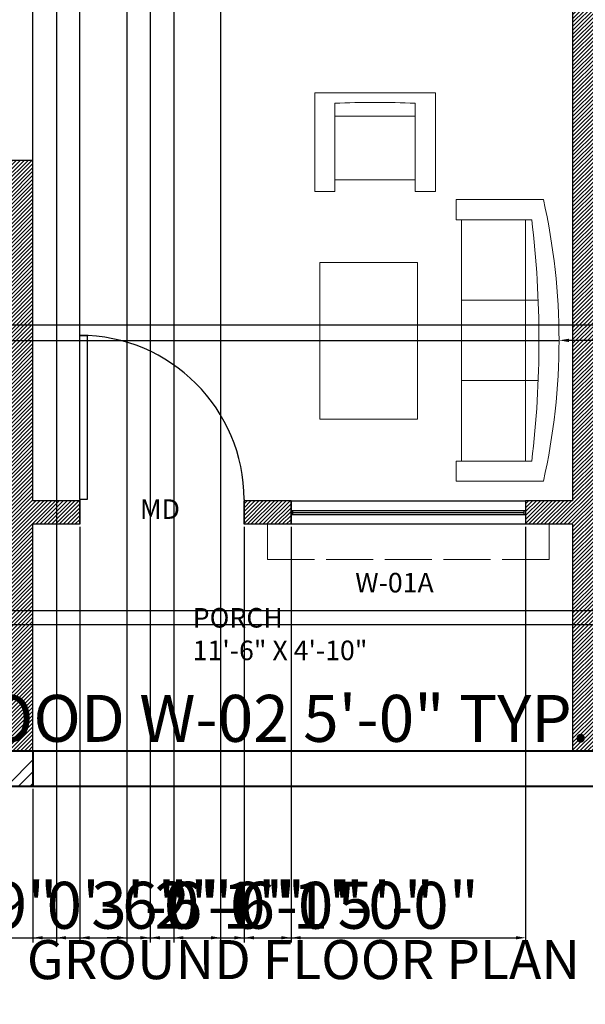
# Model space of a CAD drawing. Units: inches. Extents: x 2386 to 3029, y 792 to 1465.
# Tile 3 of 12: x 2591 to 2735, y 792 to 1044. Entities that reach past the tile are written whole.
import ezdxf

# ---------------------------------------------------------------- set-up
doc = ezdxf.new("R2010")
doc.units = ezdxf.units.IN
doc.linetypes.add('ACAD_ISO02W100', pattern=[15, 12, -3])
for name, color, linetype, lineweight in [('A-AREA-IDEN', 4, 'Continuous', 25), ('A-DIMS', 1, 'Continuous', 18), ('A-DOOR', 2, 'Continuous', 25), ('A-FURN', 6, 'Continuous', 18), ('A-TEXT', 4, 'Continuous', 25), ('A-WALL-EXT', 7, 'Continuous', 40), ('A-WALL-INT', 9, 'Continuous', 30), ('A-WALL-PATT', 9, 'Continuous', 13), ('A-WINDOW', 4, 'Continuous', 25), ('A-WINDOW-OVHD', 4, 'ACAD_ISO02W100', 18)]:
    doc.layers.add(name, color=color, linetype=linetype, lineweight=lineweight)
doc.styles.get("Standard").update_dxf_attribs({"font": 'arial.ttf'})
doc.dimstyles.new('ISO-25', dxfattribs={"dimtxt": 12, "dimasz": 2.5, "dimexe": 1.25, "dimexo": 0.625, "dimtad": 1, "dimlunit": 4, "dimtxsty": 'Standard', "dimcen": 2.5, "dimadec": 0, "dimazin": 0, "dimtfac": 1, "dimtmove": 0, "dimatfit": 3, "dimfxl": 1, "dimarcsym": 0})

# ---------------------------------------------------------------- blocks, each defined once
blk = doc.blocks.new('*U2')
for p, q in [((0, 0), (0, -6)), ((40, 0), (40, -6))]:
    blk.add_line(p, q)
blk.add_lwpolyline([(0, 0), (0, 40), (1.75, 40), (1.75, 0)], close=True)
blk.add_arc((0, 0), 40, 0, 90)
blk = doc.blocks.new('*D42')
at = {"layer": 'A-DIMS', "color": 0, "lineweight": -2, "transparency": 16777216}
for p, q in [((2504.19, 848.57), (2504.19, 858.2)), ((2506.69, 856.95), (2561.69, 856.95)), ((2564.19, 848.57), (2564.19, 858.2)), ((2564.19, 856.95), (2740.1, 856.95))]:
    blk.add_line(p, q, dxfattribs=at)
at = {"layer": 'A-DIMS', "color": 0, "transparency": 16777216}
for points in [[(2506.69, 857.36), (2506.69, 856.53), (2504.19, 856.95)], [(2561.69, 857.36), (2561.69, 856.53), (2564.19, 856.95)]]:
    blk.add_solid(points, dxfattribs=at)
at = {"layer": 'Defpoints', "color": 0, "transparency": 16777216}
for p in [(2564.19, 856.95), (2504.19, 847.95), (2564.19, 847.95)]:
    blk.add_point(p, dxfattribs=at)
at = {"layer": 'A-DIMS', "color": 0, "transparency": 16777216, "insert": (2653.39, 863.78), "char_height": 12, "attachment_point": 5}
blk.add_mtext('HOOD W-02 5\'-0" TYP.', dxfattribs=at)
blk = doc.blocks.new('*D56')
at = {"layer": 'A-DIMS', "color": 0, "lineweight": -2, "transparency": 16777216}
for p, q in [((2606.19, 914.32), (2606.19, 808)), ((2648.19, 914.32), (2648.19, 808)), ((2608.69, 809.25), (2645.69, 809.25))]:
    blk.add_line(p, q, dxfattribs=at)
at = {"layer": 'A-DIMS', "color": 0, "transparency": 16777216}
for points in [[(2608.69, 809.66), (2608.69, 808.83), (2606.19, 809.25)], [(2645.69, 809.66), (2645.69, 808.83), (2648.19, 809.25)]]:
    blk.add_solid(points, dxfattribs=at)
at = {"layer": 'Defpoints', "color": 0, "transparency": 16777216}
for p in [(2606.19, 914.95), (2648.19, 914.95), (2648.19, 809.25)]:
    blk.add_point(p, dxfattribs=at)
at = {"layer": 'A-DIMS', "color": 0, "transparency": 16777216, "insert": (2627.19, 816), "char_height": 12, "attachment_point": 5}
blk.add_mtext('3\'-6"', dxfattribs=at)
blk = doc.blocks.new('*D66')
at = {"layer": 'A-DIMS', "color": 0, "lineweight": -2, "transparency": 16777216}
for p, q in [((2630.19, 1378.32), (2630.19, 808)), ((2642.19, 1378.32), (2642.19, 808)), ((2632.69, 809.25), (2639.69, 809.25)), ((2642.19, 809.25), (2676.71, 809.25))]:
    blk.add_line(p, q, dxfattribs=at)
at = {"layer": 'A-DIMS', "color": 0, "transparency": 16777216}
for points in [[(2632.69, 809.66), (2632.69, 808.83), (2630.19, 809.25)], [(2639.69, 809.66), (2639.69, 808.83), (2642.19, 809.25)]]:
    blk.add_solid(points, dxfattribs=at)
at = {"layer": 'Defpoints', "color": 0, "transparency": 16777216}
for p in [(2630.19, 1378.95), (2642.19, 1378.95), (2642.19, 809.25)]:
    blk.add_point(p, dxfattribs=at)
at = {"layer": 'A-DIMS', "color": 0, "transparency": 16777216, "insert": (2660.7, 816), "char_height": 12, "attachment_point": 5}
blk.add_mtext('1\'-0"', dxfattribs=at)
blk = doc.blocks.new('*D70')
at = {"layer": 'A-DIMS', "color": 0, "lineweight": -2, "transparency": 16777216}
for p, q in [((2660.19, 914.32), (2660.19, 808)), ((2720.19, 914.32), (2720.19, 808)), ((2662.69, 809.25), (2717.69, 809.25))]:
    blk.add_line(p, q, dxfattribs=at)
at = {"layer": 'A-DIMS', "color": 0, "transparency": 16777216}
for points in [[(2662.69, 809.66), (2662.69, 808.83), (2660.19, 809.25)], [(2717.69, 809.66), (2717.69, 808.83), (2720.19, 809.25)]]:
    blk.add_solid(points, dxfattribs=at)
at = {"layer": 'Defpoints', "color": 0, "transparency": 16777216}
for p in [(2660.19, 914.95), (2720.19, 914.95), (2720.19, 809.25)]:
    blk.add_point(p, dxfattribs=at)
at = {"layer": 'A-DIMS', "color": 0, "transparency": 16777216, "insert": (2690.19, 816), "char_height": 12, "attachment_point": 5}
blk.add_mtext('5\'-0"', dxfattribs=at)
blk = doc.blocks.new('*D72')
at = {"layer": 'A-DIMS', "color": 0, "lineweight": -2, "transparency": 16777216}
for p, q in [((2588.19, 856.32), (2588.19, 808)), ((2594.19, 847.32), (2594.19, 808)), ((2585.69, 809.25), (2583.19, 809.25)), ((2588.19, 809.25), (2594.19, 809.25)), ((2596.69, 809.25), (2632.34, 809.25))]:
    blk.add_line(p, q, dxfattribs=at)
at = {"layer": 'A-DIMS', "color": 0, "transparency": 16777216}
for points in [[(2585.69, 809.66), (2585.69, 808.83), (2588.19, 809.25)], [(2596.69, 809.66), (2596.69, 808.83), (2594.19, 809.25)]]:
    blk.add_solid(points, dxfattribs=at)
at = {"layer": 'Defpoints', "color": 0, "transparency": 16777216}
for p in [(2588.19, 856.95), (2594.19, 847.95), (2594.19, 809.25)]:
    blk.add_point(p, dxfattribs=at)
at = {"layer": 'A-DIMS', "color": 0, "transparency": 16777216, "insert": (2615.76, 816), "char_height": 12, "attachment_point": 5}
blk.add_mtext('0\'-6"', dxfattribs=at)
blk = doc.blocks.new('*D74')
at = {"layer": 'A-DIMS', "color": 0, "lineweight": -2, "transparency": 16777216}
for p, q in [((2556.3, 889.35), (2931.14, 889.35)), ((2929.89, 886.85), (2929.89, 859.45)), ((2556.3, 856.95), (2931.14, 856.95)), ((2929.89, 856.95), (2929.89, 793.13))]:
    blk.add_line(p, q, dxfattribs=at)
at = {"layer": 'A-DIMS', "color": 0, "transparency": 16777216}
for points in [[(2929.47, 886.85), (2930.31, 886.85), (2929.89, 889.35)], [(2929.47, 859.45), (2930.31, 859.45), (2929.89, 856.95)]]:
    blk.add_solid(points, dxfattribs=at)
at = {"layer": 'Defpoints', "color": 0, "transparency": 16777216}
for p in [(2555.68, 889.35), (2555.68, 856.95), (2929.89, 856.95)]:
    blk.add_point(p, dxfattribs=at)
at = {"layer": 'A-DIMS', "color": 0, "transparency": 16777216, "insert": (2923.06, 823.79), "char_height": 12, "attachment_point": 5, "rotation": 90}
blk.add_mtext('2\'-8 1/2"', dxfattribs=at)
blk = doc.blocks.new('*D82')
at = {"layer": 'A-DIMS', "color": 0, "lineweight": -2, "transparency": 16777216}
for p, q in [((2600.19, 1306.32), (2600.19, 808)), ((2624.19, 1306.32), (2624.19, 808)), ((2602.69, 809.25), (2621.69, 809.25)), ((2624.19, 809.25), (2660.04, 809.25))]:
    blk.add_line(p, q, dxfattribs=at)
at = {"layer": 'A-DIMS', "color": 0, "transparency": 16777216}
for points in [[(2602.69, 809.66), (2602.69, 808.83), (2600.19, 809.25)], [(2621.69, 809.66), (2621.69, 808.83), (2624.19, 809.25)]]:
    blk.add_solid(points, dxfattribs=at)
at = {"layer": 'Defpoints', "color": 0, "transparency": 16777216}
for p in [(2600.19, 1306.95), (2624.19, 1306.95), (2624.19, 809.25)]:
    blk.add_point(p, dxfattribs=at)
at = {"layer": 'A-DIMS', "color": 0, "transparency": 16777216, "insert": (2643.37, 816), "char_height": 12, "attachment_point": 5}
blk.add_mtext('2\'-0"', dxfattribs=at)
blk = doc.blocks.new('*D87')
at = {"layer": 'A-DIMS', "color": 0, "lineweight": -2, "transparency": 16777216}
for p, q in [((2594.19, 921.57), (2594.19, 1427.9)), ((2606.19, 921.57), (2606.19, 1427.9)), ((2596.69, 1426.65), (2603.69, 1426.65)), ((2606.19, 1426.65), (2640.71, 1426.65))]:
    blk.add_line(p, q, dxfattribs=at)
at = {"layer": 'A-DIMS', "color": 0, "transparency": 16777216}
for points in [[(2596.69, 1427.06), (2596.69, 1426.23), (2594.19, 1426.65)], [(2603.69, 1427.06), (2603.69, 1426.23), (2606.19, 1426.65)]]:
    blk.add_solid(points, dxfattribs=at)
at = {"layer": 'Defpoints', "color": 0, "transparency": 16777216}
for p in [(2606.19, 1426.65), (2594.19, 920.95), (2606.19, 920.95)]:
    blk.add_point(p, dxfattribs=at)
at = {"layer": 'A-DIMS', "color": 0, "transparency": 16777216, "insert": (2624.7, 1433.4), "char_height": 12, "attachment_point": 5}
blk.add_mtext('1\'-0"', dxfattribs=at)
blk = doc.blocks.new('*D88')
at = {"layer": 'A-DIMS', "color": 0, "lineweight": -2, "transparency": 16777216}
for p, q in [((2648.19, 914.32), (2648.19, 808)), ((2660.19, 914.32), (2660.19, 808)), ((2650.69, 809.25), (2657.69, 809.25)), ((2660.19, 809.25), (2694.71, 809.25))]:
    blk.add_line(p, q, dxfattribs=at)
at = {"layer": 'A-DIMS', "color": 0, "transparency": 16777216}
for points in [[(2650.69, 809.66), (2650.69, 808.83), (2648.19, 809.25)], [(2657.69, 809.66), (2657.69, 808.83), (2660.19, 809.25)]]:
    blk.add_solid(points, dxfattribs=at)
at = {"layer": 'Defpoints', "color": 0, "transparency": 16777216}
for p in [(2648.19, 914.95), (2660.19, 914.95), (2660.19, 809.25)]:
    blk.add_point(p, dxfattribs=at)
at = {"layer": 'A-DIMS', "color": 0, "transparency": 16777216, "insert": (2678.7, 816), "char_height": 12, "attachment_point": 5}
blk.add_mtext('1\'-0"', dxfattribs=at)
blk = doc.blocks.new('*D92')
at = {"layer": 'A-DIMS', "color": 0, "lineweight": -2, "transparency": 16777216}
for p, q in [((2618.19, 1145.32), (2618.19, 808)), ((2624.19, 1145.32), (2624.19, 808)), ((2615.69, 809.25), (2613.19, 809.25)), ((2618.19, 809.25), (2624.19, 809.25)), ((2626.69, 809.25), (2662.34, 809.25))]:
    blk.add_line(p, q, dxfattribs=at)
at = {"layer": 'A-DIMS', "color": 0, "transparency": 16777216}
for points in [[(2615.69, 809.66), (2615.69, 808.83), (2618.19, 809.25)], [(2626.69, 809.66), (2626.69, 808.83), (2624.19, 809.25)]]:
    blk.add_solid(points, dxfattribs=at)
at = {"layer": 'Defpoints', "color": 0, "transparency": 16777216}
for p in [(2618.19, 1145.95), (2624.19, 1145.95), (2624.19, 809.25)]:
    blk.add_point(p, dxfattribs=at)
at = {"layer": 'A-DIMS', "color": 0, "transparency": 16777216, "insert": (2645.76, 816), "char_height": 12, "attachment_point": 5}
blk.add_mtext('0\'-6"', dxfattribs=at)
blk = doc.blocks.new('*D97')
at = {"layer": 'A-DIMS', "color": 0, "lineweight": -2, "transparency": 16777216}
for p, q in [((2516.82, 965.95), (2931.14, 965.95)), ((2929.89, 895.45), (2929.89, 963.45)), ((2516.82, 892.95), (2931.14, 892.95))]:
    blk.add_line(p, q, dxfattribs=at)
at = {"layer": 'A-DIMS', "color": 0, "transparency": 16777216}
for points in [[(2929.47, 963.45), (2930.31, 963.45), (2929.89, 965.95)], [(2929.47, 895.45), (2930.31, 895.45), (2929.89, 892.95)]]:
    blk.add_solid(points, dxfattribs=at)
at = {"layer": 'Defpoints', "color": 0, "transparency": 16777216}
for p in [(2516.19, 965.95), (2929.89, 965.95), (2516.19, 892.95)]:
    blk.add_point(p, dxfattribs=at)
at = {"layer": 'A-DIMS', "color": 0, "transparency": 16777216, "insert": (2923.14, 929.45), "char_height": 12, "attachment_point": 5, "rotation": 90}
blk.add_mtext('6\'-1"', dxfattribs=at)
blk = doc.blocks.new('*D99')
at = {"layer": 'A-DIMS', "color": 0, "lineweight": -2, "transparency": 16777216}
for p, q in [((2530.41, 1210.29), (2530.41, 808)), ((2563.26, 1210.63), (2563.26, 808)), ((2532.91, 809.25), (2560.76, 809.25)), ((2563.26, 809.25), (2599.11, 809.25))]:
    blk.add_line(p, q, dxfattribs=at)
at = {"layer": 'A-DIMS', "color": 0, "transparency": 16777216}
for points in [[(2532.91, 809.66), (2532.91, 808.83), (2530.41, 809.25)], [(2560.76, 809.66), (2560.76, 808.83), (2563.26, 809.25)]]:
    blk.add_solid(points, dxfattribs=at)
at = {"layer": 'Defpoints', "color": 0, "transparency": 16777216}
for p in [(2530.41, 1210.91), (2563.26, 1211.26), (2563.26, 809.25)]:
    blk.add_point(p, dxfattribs=at)
at = {"layer": 'A-DIMS', "color": 0, "transparency": 16777216, "insert": (2582.43, 816), "char_height": 12, "attachment_point": 5}
blk.add_mtext('2\'-9"', dxfattribs=at)
blk = doc.blocks.new('*D104')
at = {"layer": 'A-DIMS', "color": 0, "lineweight": -2, "transparency": 16777216}
for p, q in [((2564.73, 961.97), (2728.73, 961.97)), ((2854.11, 961.97), (2731.23, 961.97))]:
    blk.add_line(p, q, dxfattribs=at)
at = {"layer": 'A-DIMS', "color": 0, "transparency": 16777216}
blk.add_solid([(2731.23, 962.38), (2731.23, 961.55), (2728.73, 961.97)], dxfattribs=at)
at = {"layer": 'Defpoints', "color": 0, "transparency": 16777216}
for p in [(2564.73, 961.97), (2728.73, 961.97)]:
    blk.add_point(p, dxfattribs=at)
at = {"layer": 'A-DIMS', "color": 0, "transparency": 16777216, "insert": (2827.13, 968.72), "char_height": 12, "attachment_point": 5, "rotation": 359.9999}
blk.add_mtext('R13\'-8"', dxfattribs=at)

msp = doc.modelspace()

# ---------------------------------------------------------------- hatches: boundary and pattern name
at = {"layer": 'A-WALL-PATT'}
h = msp.add_hatch(dxfattribs=at)
h.set_pattern_fill('GOST_GROUND', color=256)
h.paths.add_polyline_path([(2480.19, 1276.948), (2471.19, 1276.948), (2471.19, 1211.948), (2480.19, 1211.948)])
h.paths.add_polyline_path([(2480.19, 1378.948), (2510.19, 1378.948), (2510.19, 1378.969), (2523.779, 1378.969), (2580.602, 1378.959), (2580.602, 1378.969), (2594.19, 1378.969), (2642.19, 1378.948), (2642.19, 1387.948), (2471.19, 1387.948), (2471.19, 1336.948), (2480.19, 1336.948)])
h.paths.add_polyline_path([(2891.19, 1387.948), (2666.19, 1387.948), (2666.19, 1378.948), (2882.19, 1378.948), (2882.19, 1355.948), (2891.19, 1355.948)])
h.paths.add_polyline_path([(2891.19, 1331.948), (2882.19, 1331.948), (2882.19, 1331.449), (2882.19, 1261.948), (2891.19, 1261.948)])
h.paths.add_polyline_path([(2891.19, 1201.948), (2882.19, 1201.948), (2882.19, 1189.948), (2882.19, 1159.948), (2882.19, 1117.948), (2891.19, 1117.948)])
h.paths.add_polyline_path([(2891.19, 1057.948), (2882.19, 1057.948), (2882.19, 856.948), (2882.19, 847.948), (2891.19, 847.948)])
h.paths.add_polyline_path([(2594.19, 856.948), (2558.19, 856.948), (2558.19, 847.948), (2594.19, 847.948)])
h.paths.add_polyline_path([(2510.19, 856.948), (2480.19, 856.948), (2480.19, 905.448), (2471.19, 905.448), (2471.19, 847.948), (2510.19, 847.948)])
h.paths.add_polyline_path([(2480.19, 1007.948), (2471.19, 1007.948), (2471.19, 953.448), (2480.19, 953.448)])
h.paths.add_polyline_path([(2480.19, 1103.948), (2471.19, 1103.948), (2471.19, 1043.948), (2480.19, 1043.948)])
h = msp.add_hatch(dxfattribs=at)
h.set_pattern_fill('JIS_WOOD', color=256)
h.paths.add_polyline_path([(2624.19, 1229.948), (2624.19, 1145.948), (2618.19, 1145.948), (2618.19, 1140.548), (2618.19, 1139.948), (2630.19, 1139.948), (2630.19, 1240.948), (2624.19, 1240.948), (2624.19, 1234.948), (2480.19, 1234.948), (2480.19, 1229.948)])
h.paths.add_polyline_path([(2582.19, 1139.948), (2582.19, 1145.948), (2480.19, 1145.948), (2480.19, 1139.948)], flags=17)
h.paths.add_polyline_path([(2480.19, 1007.948), (2480.19, 1001.948), (2546.19, 1001.948), (2546.19, 1007.348), (2546.19, 1007.948)])
h.paths.add_polyline_path([(2594.19, 1007.948), (2582.19, 1007.948), (2582.19, 1001.948), (2588.19, 1001.948), (2588.19, 856.948), (2594.19, 856.948), (2594.19, 914.948), (2606.19, 914.948), (2606.19, 920.948), (2594.19, 920.948)])
h.paths.add_polyline_path([(2738.19, 1015.948), (2882.19, 1015.948), (2882.19, 1021.948), (2738.19, 1021.948), (2738.19, 1111.948), (2732.19, 1111.948), (2732.19, 920.948), (2720.19, 920.948), (2720.19, 914.948), (2732.19, 914.948), (2732.19, 856.948), (2738.19, 856.948)])
h.paths.add_polyline_path([(2660.19, 914.948), (2660.19, 920.948), (2648.19, 920.948), (2648.19, 914.948)])
h.paths.add_polyline_path([(2738.19, 1159.948), (2738.19, 1165.948), (2737.59, 1165.948), (2732.19, 1165.948), (2732.19, 1147.948), (2737.59, 1147.948), (2738.19, 1147.948), (2738.19, 1153.948), (2882.19, 1153.948), (2882.19, 1159.948)])
h.paths.add_polyline_path([(2732.19, 1201.948), (2738.19, 1201.948), (2738.19, 1303.948), (2774.19, 1303.948), (2774.19, 1308.948), (2768.19, 1308.948), (2768.19, 1378.948), (2762.19, 1378.948), (2762.19, 1308.948), (2726.19, 1308.948), (2726.19, 1303.948), (2732.19, 1303.948)])
h.paths.add_polyline_path([(2696.19, 1303.948), (2696.19, 1308.948), (2630.19, 1308.948), (2630.19, 1378.948), (2624.19, 1378.948), (2624.19, 1276.948), (2630.19, 1276.948), (2630.19, 1303.948)])

# ---------------------------------------------------------------- linework, layer by layer
at = {"layer": 'A-FURN'}
for p, q in [((2666.25, 1025.273), (2666.25, 999.987)), ((2697.107, 1025.273), (2666.25, 1025.273)), ((2697.107, 999.987), (2697.107, 1025.273)), ((2671.393, 999.987), (2671.393, 1022.592)), ((2691.964, 999.987), (2691.964, 1022.592)), ((2691.964, 1019.324), (2671.393, 1019.324)), ((2691.964, 1002.987), (2671.393, 1002.987)), ((2666.25, 999.987), (2671.393, 999.987)), ((2691.964, 999.987), (2697.107, 999.987)), ((2702.444, 997.967), (2724.73, 997.967)), ((2702.444, 992.824), (2702.444, 997.967)), ((2702.444, 992.824), (2721.756, 992.824)), ((2703.779, 992.824), (2703.779, 931.11)), ((2720.117, 992.824), (2720.117, 931.11)), ((2692.557, 981.862), (2667.557, 981.862)), ((2667.557, 981.862), (2667.557, 941.862)), ((2692.557, 941.862), (2692.557, 981.862)), ((2703.779, 972.253), (2723.384, 972.253)), ((2703.779, 951.682), (2723.384, 951.682)), ((2667.557, 941.862), (2692.557, 941.862)), ((2702.444, 931.11), (2721.756, 931.11)), ((2702.444, 925.967), (2702.444, 931.11)), ((2724.73, 925.967), (2702.444, 925.967))]:
    msp.add_line(p, q, dxfattribs=at)
for centre, radius, start, end in [((2681.679, 761.939), 260.855, 87.74019, 92.25979), ((2564.73, 961.967), 164, 347.31962, 12.68039), ((2462.731, 961.967), 260.855, 353.2065, 6.79353)]:
    msp.add_arc(centre, radius, start, end, dxfattribs=at)
at = {"layer": 'A-WALL-EXT'}
for p, q in [((2882.19, 856.948), (2558.19, 856.948)), ((2594.19, 856.948), (2594.19, 847.948)), ((2891.19, 847.948), (2558.19, 847.948))]:
    msp.add_line(p, q, dxfattribs=at)
at = {"layer": 'A-WALL-INT'}
for p, q in [((2732.19, 1111.948), (2732.19, 920.948)), ((2594.19, 1007.948), (2582.19, 1007.948)), ((2594.19, 920.948), (2594.19, 1007.948)), ((2606.19, 920.948), (2594.19, 920.948)), ((2606.19, 914.948), (2606.19, 920.948)), ((2648.19, 914.948), (2648.19, 920.948)), ((2660.19, 920.948), (2648.19, 920.948)), ((2660.19, 914.948), (2660.19, 920.948)), ((2732.19, 920.948), (2720.19, 920.948)), ((2720.19, 920.948), (2720.19, 914.948)), ((2594.19, 856.948), (2594.19, 914.948)), ((2606.19, 914.948), (2594.19, 914.948)), ((2660.19, 914.948), (2648.19, 914.948)), ((2732.19, 914.948), (2720.19, 914.948)), ((2732.19, 914.948), (2732.19, 856.948))]:
    msp.add_line(p, q, dxfattribs=at)
at = {"layer": 'A-WINDOW'}
for p, q in [((2660.19, 920.948), (2720.19, 920.948)), ((2660.19, 920.948), (2660.19, 914.948)), ((2720.19, 920.948), (2720.19, 914.948)), ((2660.19, 918.448), (2720.19, 918.448)), ((2660.19, 917.448), (2720.19, 917.448)), ((2660.69, 917.448), (2660.69, 918.448)), ((2660.69, 917.948), (2719.69, 917.948)), ((2719.69, 918.448), (2719.69, 917.448)), ((2720.19, 914.948), (2660.19, 914.948))]:
    msp.add_line(p, q, dxfattribs=at)
at = {"layer": 'A-WINDOW-OVHD'}
for p, q in [((2654.19, 914.948), (2654.19, 905.948)), ((2726.19, 914.948), (2726.19, 905.948)), ((2654.19, 905.948), (2726.19, 905.948))]:
    msp.add_line(p, q, dxfattribs=at)

# ---------------------------------------------------------------- block references
at = {"layer": 'A-DOOR', "xscale": 1.05, "yscale": 1.05, "zscale": 1.05}
msp.add_blockref('*U2', (2606.19, 921.248), dxfattribs=at)

# ---------------------------------------------------------------- texts
at = {"layer": 'A-AREA-IDEN', "insert": (2635.059, 893.547), "char_height": 5, "attachment_point": 1}
msp.add_mtext_dynamic_manual_height_columns('PORCH\\P11\'-6" X 4\'-10"', width=52.37406, gutter_width=12.5, heights=[0], dxfattribs=at)
at = {"layer": 'A-TEXT', "attachment_point": 1}
for s, width, insert, char_height in [('MD', 38.22215, (2621.549, 921.326), 5), ('W-01A', 38.22215, (2676.604, 902.527), 5), ('GROUND FLOOR PLAN', 161.12866, (2592.643, 808.665), 10)]:
    msp.add_mtext_dynamic_manual_height_columns(s, width=width, gutter_width=12.5, heights=[0], dxfattribs=dict(at, insert=insert, char_height=char_height))

# ---------------------------------------------------------------- dimensions: what is measured, and where the dimension line sits
at = {"layer": 'A-DIMS'}
for base, p1, p2, picture, middle in [((2606.19, 1426.648), (2594.19, 920.948), (2606.19, 920.948), '*D87', (2624.7, 1433.4)), ((2642.19, 809.248), (2630.19, 1378.948), (2642.19, 1378.948), '*D66', (2660.7, 816)), ((2624.19, 809.248), (2600.19, 1306.948), (2624.19, 1306.948), '*D82', (2643.367, 816)), ((2563.257, 809.248), (2530.413, 1210.915), (2563.257, 1211.257), '*D99', (2582.434, 816)), ((2624.19, 809.248), (2618.19, 1145.948), (2624.19, 1145.948), '*D92', (2645.765, 816)), ((2648.19, 809.248), (2606.19, 914.948), (2648.19, 914.948), '*D56', (2627.19, 816.004)), ((2660.19, 809.248), (2648.19, 914.948), (2660.19, 914.948), '*D88', (2678.7, 816)), ((2720.19, 809.248), (2660.19, 914.948), (2720.19, 914.948), '*D70', (2690.19, 816)), ((2594.19, 809.248), (2588.19, 856.948), (2594.19, 847.948), '*D72', (2615.765, 816))]:
    dim = msp.add_linear_dim(base=base, p1=p1, p2=p2, dimstyle='ISO-25', override={"dimdec": 1, "dimlfac": 1, "dimrnd": 0, "dimzin": 1, "dimdsep": 46, "dimlunit": 4, "dimfrac": 2}, dxfattribs=at)
    dim.commit()
    dim.dimension.update_dxf_attribs({"geometry": picture, "text_midpoint": middle})
dim = msp.add_radius_dim(center=(2564.73, 961.967), mpoint=(2728.73, 961.967), dimstyle='ISO-25', override={"dimdec": 1, "dimlfac": 1, "dimrnd": 0, "dimzin": 1, "dimdsep": 46, "dimlunit": 4, "dimfrac": 2}, dxfattribs=at)
dim.commit()
dim.dimension.update_dxf_attribs({"geometry": '*D104', "text_midpoint": (2827.13, 961.967), "dimtype": 164})
for base, p1, p2, picture, middle in [((2929.89, 965.948), (2516.19, 892.948), (2516.19, 965.948), '*D97', (2923.138, 929.448)), ((2929.89, 856.948), (2555.676, 889.348), (2555.676, 856.948), '*D74', (2923.06, 823.79))]:
    dim = msp.add_linear_dim(base=base, p1=p1, p2=p2, angle=90, dimstyle='ISO-25', override={"dimdec": 1, "dimlfac": 1, "dimrnd": 0, "dimzin": 1, "dimdsep": 46, "dimlunit": 4, "dimfrac": 2}, dxfattribs=at)
    dim.commit()
    dim.dimension.update_dxf_attribs({"geometry": picture, "text_midpoint": middle})
dim = msp.add_linear_dim(base=(2564.19, 856.948), p1=(2504.19, 847.948), p2=(2564.19, 847.948), text='HOOD W-02 <> TYP.', dimstyle='ISO-25', override={"dimdec": 1, "dimlfac": 1, "dimrnd": 0, "dimzin": 1, "dimdsep": 46, "dimlunit": 4, "dimfrac": 2}, dxfattribs=at)
dim.commit()
dim.dimension.update_dxf_attribs({"geometry": '*D42', "text_midpoint": (2653.394, 863.782)})

doc.saveas('drawing.dxf')
